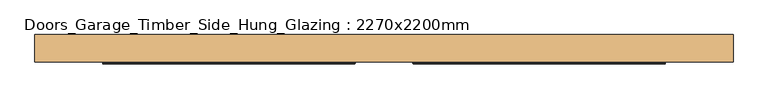
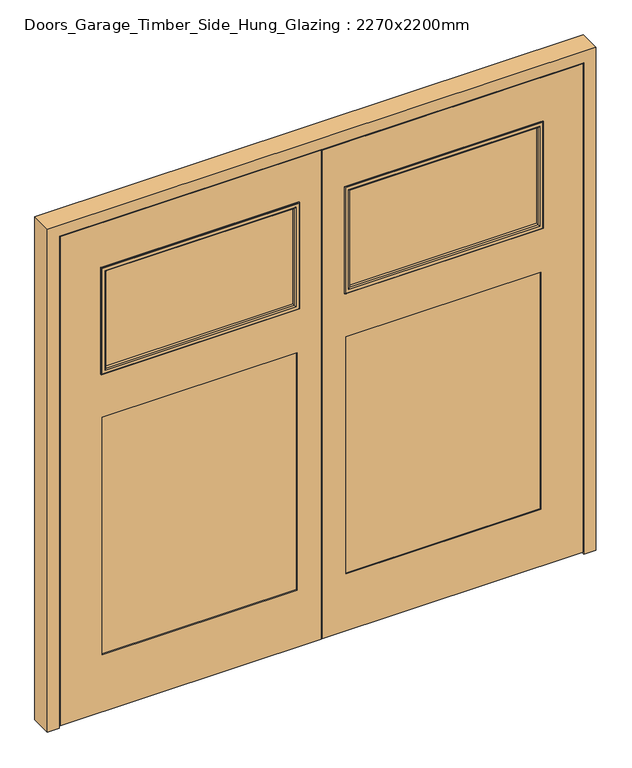
"""IFC4 building model written with IfcOpenShell, lengths in millimetres: door geometry, Doors_Garage_Timber_Side_Hung_Glazing : 2270x2200mm."""

from ifc_helpers import new_model, si_unit, frame, origin, place, context, project, spatial, polyline, ellipse_curve, outline, extrude, faceted_brep, source, transform, mapped, element, save
from ifc_brep_helpers import plane_surface, cylinder_surface, advanced_brep


def doors_garage_timber_side_hung_glazing_2270x2200mm_badb7014(model_context):
    return source(origin(), model_context, "Body", "SolidModel", [
        faceted_brep([(1085.0, -76.6, 0.0), (1085.0, -41.6, 0.0), (1063.0, -41.6, 0.0), (1063.0, 12.4, 0.0), (1135.0, 12.4, 0.0), (1135.0, -76.6, 0.0), (1135.0, -76.6, 2200.0), (-1135.0, -76.6, 2200.0), (-1135.0, -76.6, 0.0), (-1085.0, -76.6, 0.0), (-1085.0, -76.6, 2150.0), (1085.0, -76.6, 2150.0), (1135.0, 12.4, 2200.0), (1063.0, 12.4, 2128.0), (-1063.0, 12.4, 2128.0), (-1063.0, 12.4, 0.0), (-1135.0, 12.4, 0.0), (-1135.0, 12.4, 2200.0), (1063.0, -41.6, 2128.0), (1085.0, -41.6, 2150.0), (-1085.0, -41.6, 2150.0), (-1085.0, -41.6, 0.0), (-1063.0, -41.6, 0.0), (-1063.0, -41.6, 2128.0)], [[[0, 1, 2, 3, 4, 5]], [[5, 6, 7, 8, 9, 10, 11, 0]], [[4, 12, 6, 5]], [[3, 13, 14, 15, 16, 17, 12, 4]], [[2, 18, 13, 3]], [[1, 19, 20, 21, 22, 23, 18, 2]], [[0, 11, 19, 1]], [[9, 21, 20, 10]], [[8, 16, 15, 22, 21, 9]], [[7, 17, 16, 8]], [[14, 23, 22, 15]], [[6, 12, 17, 7]], [[13, 18, 23, 14]], [[10, 20, 19, 11]]]),
        faceted_brep([(1.5, -44.6, 10.0), (1.5, -44.6, 2147.0), (1082.0, -44.6, 2147.0), (1082.0, -44.6, 10.0), (101.5, -44.6, 1947.0), (101.5, -44.6, 1497.0), (907.0, -44.6, 1497.0), (907.0, -44.6, 1947.0), (1.5, -76.6, 10.0), (1082.0, -76.6, 10.0), (1082.0, -76.6, 2147.0), (1.5, -76.6, 2147.0), (101.5, -76.6, 1947.0), (907.0, -76.6, 1947.0), (907.0, -76.6, 1497.0), (101.5, -76.6, 1497.0), (101.5, -76.6, 1297.0), (907.0, -76.6, 1297.0), (907.0, -76.6, 260.0), (101.5, -76.6, 260.0), (101.5, -71.6, 260.0), (907.0, -71.6, 260.0), (907.0, -71.6, 1297.0), (101.5, -71.6, 1297.0)], [[[0, 1, 2, 3], [4, 5, 6, 7]], [[8, 9, 10, 11], [12, 13, 14, 15], [16, 17, 18, 19]], [[3, 9, 8, 0]], [[2, 10, 9, 3]], [[1, 11, 10, 2]], [[0, 8, 11, 1]], [[7, 13, 12, 4]], [[6, 14, 13, 7]], [[5, 15, 14, 6]], [[4, 12, 15, 5]], [[20, 21, 22, 23]], [[23, 16, 19, 20]], [[22, 17, 16, 23]], [[21, 18, 17, 22]], [[20, 19, 18, 21]]]),
        faceted_brep([(-1082.0, -44.6, 10.0), (-1082.0, -44.6, 2147.0), (-1.5, -44.6, 2147.0), (-1.5, -44.6, 10.0), (-101.5, -44.6, 1497.0), (-101.5, -44.6, 1947.0), (-907.0, -44.6, 1947.0), (-907.0, -44.6, 1497.0), (-1082.0, -76.6, 10.0), (-1.5, -76.6, 10.0), (-1.5, -76.6, 2147.0), (-1082.0, -76.6, 2147.0), (-101.5, -76.6, 1497.0), (-907.0, -76.6, 1497.0), (-907.0, -76.6, 1947.0), (-101.5, -76.6, 1947.0), (-101.5, -76.6, 1297.0), (-101.5, -76.6, 260.0), (-907.0, -76.6, 260.0), (-907.0, -76.6, 1297.0), (-907.0, -71.6, 1297.0), (-907.0, -71.6, 260.0), (-101.5, -71.6, 260.0), (-101.5, -71.6, 1297.0)], [[[0, 1, 2, 3], [4, 5, 6, 7]], [[8, 9, 10, 11], [12, 13, 14, 15], [16, 17, 18, 19]], [[3, 9, 8, 0]], [[2, 10, 9, 3]], [[1, 11, 10, 2]], [[0, 8, 11, 1]], [[7, 13, 12, 4]], [[6, 14, 13, 7]], [[5, 15, 14, 6]], [[4, 12, 15, 5]], [[20, 21, 22, 23]], [[23, 16, 19, 20]], [[22, 17, 16, 23]], [[21, 18, 17, 22]], [[20, 19, 18, 21]]]),
        extrude(outline(polyline([(907.0, -54.6), (907.0, -66.6), (101.5, -66.6), (101.5, -54.6), (907.0, -54.6)])), frame((0.0, 0.0, 1497.0), z_axis=(0.0, 0.0, 1.0), x_axis=(1.0, 0.0, 0.0)), (0.0, 0.0, 1.0), 450.0),
        extrude(outline(polyline([(-101.5, -54.6), (-101.5, -66.6), (-907.0, -66.6), (-907.0, -54.6), (-101.5, -54.6)])), frame((0.0, 0.0, 1497.0), z_axis=(0.0, 0.0, 1.0), x_axis=(1.0, 0.0, 0.0)), (0.0, 0.0, 1.0), 450.0),
        advanced_brep(
        [(-907.0, -66.6, 1947.0), (-907.0, -66.6, 1497.0), (-907.0, -76.6, 1497.0), (-907.0, -76.6, 1947.0), (-895.0, -77.6, 1935.0), (-895.0, -77.6, 1509.0), (-895.0, -66.6, 1509.0), (-895.0, -66.6, 1935.0), (-900.0, -82.6, 1940.0), (-900.0, -82.6, 1504.0), (-915.0, -80.6, 1955.0), (-915.0, -80.6, 1489.0), (-913.0, -82.6, 1491.0), (-913.0, -82.6, 1953.0), (-915.0, -76.6, 1955.0), (-915.0, -76.6, 1489.0), (-101.5, -66.6, 1497.0), (-101.5, -76.6, 1497.0), (-113.5, -77.6, 1509.0), (-113.5, -66.6, 1509.0), (-108.5, -82.6, 1504.0), (-93.5, -80.6, 1489.0), (-95.5, -82.6, 1491.0), (-93.5, -76.6, 1489.0), (-101.5, -66.6, 1947.0), (-101.5, -76.6, 1947.0), (-113.5, -77.6, 1935.0), (-113.5, -66.6, 1935.0), (-108.5, -82.6, 1940.0), (-93.5, -80.6, 1955.0), (-95.5, -82.6, 1953.0), (-93.5, -76.6, 1955.0)],
        [
            (0, 1),
            (1, 2),
            (2, 3),
            (3, 0),
            (4, 5),
            (5, 6),
            (6, 7),
            (7, 4),
            (8, 9),
            (9, 5, ellipse_curve(frame((-900.0, -77.6, 1504.0), z_axis=(-0.7071067811865475, 0.0, 0.7071067811865475), x_axis=(0.7071067811865474, 0.0, 0.7071067811865476)), 7.0710678, 5.0)),
            (4, 8, ellipse_curve(frame((-900.0, -77.6, 1940.0), z_axis=(-0.7071067811865475, 0.0, -0.7071067811865475), x_axis=(-0.7071067811865474, 0.0, 0.7071067811865476)), 7.0710678, 5.0)),
            (10, 11),
            (11, 12, ellipse_curve(frame((-913.0, -80.6, 1491.0), z_axis=(-0.7071067811865475, 0.0, 0.7071067811865475), x_axis=(0.7071067811865474, 0.0, 0.7071067811865476)), 2.8284271, 2.0)),
            (12, 13),
            (13, 10, ellipse_curve(frame((-913.0, -80.6, 1953.0), z_axis=(-0.7071067811865475, 0.0, -0.7071067811865475), x_axis=(-0.7071067811865474, 0.0, 0.7071067811865476)), 2.8284271, 2.0)),
            (14, 15),
            (15, 11),
            (10, 14),
            (1, 16),
            (16, 17),
            (17, 2),
            (5, 18),
            (18, 19),
            (19, 6),
            (9, 20),
            (20, 18, ellipse_curve(frame((-108.5, -77.6, 1504.0), z_axis=(-0.7071067811865475, 0.0, -0.7071067811865475), x_axis=(-0.7071067811865476, 0.0, 0.7071067811865474)), 7.0710678, 5.0)),
            (11, 21),
            (21, 22, ellipse_curve(frame((-95.5, -80.6, 1491.0), z_axis=(-0.7071067811865475, 0.0, -0.7071067811865475), x_axis=(-0.7071067811865476, 0.0, 0.7071067811865474)), 2.8284271, 2.0)),
            (22, 12),
            (15, 23),
            (23, 21),
            (16, 24),
            (24, 25),
            (25, 17),
            (18, 26),
            (26, 27),
            (27, 19),
            (20, 28),
            (28, 26, ellipse_curve(frame((-108.5, -77.6, 1940.0), z_axis=(0.7071067811865475, 0.0, -0.7071067811865475), x_axis=(-0.7071067811865474, 0.0, -0.7071067811865476)), 7.0710678, 5.0)),
            (21, 29),
            (29, 30, ellipse_curve(frame((-95.5, -80.6, 1953.0), z_axis=(0.7071067811865475, 0.0, -0.7071067811865475), x_axis=(-0.7071067811865474, 0.0, -0.7071067811865476)), 2.8284271, 2.0)),
            (30, 22),
            (23, 31),
            (31, 29),
            (14, 31),
            (25, 3),
            (24, 0),
            (27, 7),
            (26, 4),
            (28, 8),
            (30, 13),
            (29, 10),
        ],
        [
            plane_surface(frame((-907.0, -76.6, 1947.0), z_axis=(-1.0, 0.0, 0.0), x_axis=(0.0, 0.0, -1.0))),
            plane_surface(frame((-895.0, -66.6, 1935.0), z_axis=(1.0, 0.0, 0.0), x_axis=(0.0, 0.0, -1.0))),
            cylinder_surface(frame((-900.0, -77.6, 1947.0), z_axis=(0.0, 0.0, 1.0), x_axis=(-1.0, 0.0, 0.0)), 5.0),
            cylinder_surface(frame((-913.0, -80.6, 1947.0), z_axis=(0.0, 0.0, 1.0), x_axis=(-1.0, 0.0, 0.0)), 2.0),
            plane_surface(frame((-915.0, -80.6, 1955.0), z_axis=(-1.0, 0.0, 0.0), x_axis=(0.0, 0.0, -1.0))),
            plane_surface(frame((-907.0, -76.6, 1497.0), z_axis=(0.0, 0.0, -1.0), x_axis=(1.0, 0.0, 0.0))),
            plane_surface(frame((-895.0, -66.6, 1509.0), z_axis=(0.0, 0.0, 1.0), x_axis=(1.0, 0.0, 0.0))),
            cylinder_surface(frame((-907.0, -77.6, 1504.0), z_axis=(-1.0, 0.0, 0.0), x_axis=(0.0, 0.0, -1.0)), 5.0),
            cylinder_surface(frame((-907.0, -80.6, 1491.0), z_axis=(-1.0, 0.0, 0.0), x_axis=(0.0, 0.0, -1.0)), 2.0),
            plane_surface(frame((-915.0, -80.6, 1489.0), z_axis=(0.0, 0.0, -1.0), x_axis=(1.0, 0.0, 0.0))),
            plane_surface(frame((-101.5, -76.6, 1497.0), z_axis=(1.0, 0.0, 0.0), x_axis=(0.0, 0.0, 1.0))),
            plane_surface(frame((-113.5, -66.6, 1509.0), z_axis=(-1.0, 0.0, 0.0), x_axis=(0.0, 0.0, 1.0))),
            cylinder_surface(frame((-108.5, -77.6, 1497.0), z_axis=(0.0, 0.0, -1.0), x_axis=(1.0, 0.0, 0.0)), 5.0),
            cylinder_surface(frame((-95.5, -80.6, 1497.0), z_axis=(0.0, 0.0, -1.0), x_axis=(1.0, 0.0, 0.0)), 2.0),
            plane_surface(frame((-93.5, -80.6, 1489.0), z_axis=(1.0, 0.0, 0.0), x_axis=(0.0, 0.0, 1.0))),
            plane_surface(frame((-93.5, -76.6, 1955.0), z_axis=(0.0, 1.0, 0.0), x_axis=(-1.0, 0.0, 0.0))),
            plane_surface(frame((-101.5, -76.6, 1947.0), z_axis=(0.0, 0.0, 1.0), x_axis=(-1.0, 0.0, 0.0))),
            plane_surface(frame((-101.5, -66.6, 1947.0), z_axis=(0.0, 1.0, 0.0), x_axis=(-1.0, 0.0, 0.0))),
            plane_surface(frame((-113.5, -66.6, 1935.0), z_axis=(0.0, 0.0, -1.0), x_axis=(-1.0, 0.0, 0.0))),
            cylinder_surface(frame((-101.5, -77.6, 1940.0), z_axis=(1.0, 0.0, 0.0), x_axis=(0.0, 0.0, 1.0)), 5.0),
            plane_surface(frame((-108.5, -82.6, 1940.0), z_axis=(0.0, -1.0, 0.0), x_axis=(-1.0, 0.0, 0.0))),
            cylinder_surface(frame((-101.5, -80.6, 1953.0), z_axis=(1.0, 0.0, 0.0), x_axis=(0.0, 0.0, 1.0)), 2.0),
            plane_surface(frame((-93.5, -80.6, 1955.0), z_axis=(0.0, 0.0, 1.0), x_axis=(-1.0, 0.0, 0.0))),
        ],
        [
            (0, [[1, 2, 3, 4]]),
            (1, [[5, 6, 7, 8]]),
            (2, [[9, 10, -5, 11]]),
            (3, [[12, 13, 14, 15]]),
            (4, [[16, 17, -12, 18]]),
            (5, [[19, 20, 21, -2]]),
            (6, [[22, 23, 24, -6]]),
            (7, [[25, 26, -22, -10]]),
            (8, [[27, 28, 29, -13]]),
            (9, [[30, 31, -27, -17]]),
            (10, [[32, 33, 34, -20]]),
            (11, [[35, 36, 37, -23]]),
            (12, [[38, 39, -35, -26]]),
            (13, [[40, 41, 42, -28]]),
            (14, [[43, 44, -40, -31]]),
            (15, [[-16, 45, -43, -30], [-3, -21, -34, 46]]),
            (16, [[47, -4, -46, -33]]),
            (17, [[-1, -47, -32, -19], [-7, -24, -37, 48]]),
            (18, [[49, -8, -48, -36]]),
            (19, [[50, -11, -49, -39]]),
            (20, [[-14, -29, -42, 51], [-9, -50, -38, -25]]),
            (21, [[52, -15, -51, -41]]),
            (22, [[-45, -18, -52, -44]]),
        ],
    ),
        advanced_brep(
        [(101.5, -66.6, 1947.0), (101.5, -66.6, 1497.0), (101.5, -76.6, 1497.0), (101.5, -76.6, 1947.0), (113.5, -77.6, 1935.0), (113.5, -77.6, 1509.0), (113.5, -66.6, 1509.0), (113.5, -66.6, 1935.0), (108.5, -82.6, 1940.0), (108.5, -82.6, 1504.0), (93.5, -80.6, 1955.0), (93.5, -80.6, 1489.0), (95.5, -82.6, 1491.0), (95.5, -82.6, 1953.0), (93.5, -76.6, 1955.0), (93.5, -76.6, 1489.0), (907.0, -66.6, 1497.0), (907.0, -76.6, 1497.0), (895.0, -77.6, 1509.0), (895.0, -66.6, 1509.0), (900.0, -82.6, 1504.0), (915.0, -80.6, 1489.0), (913.0, -82.6, 1491.0), (915.0, -76.6, 1489.0), (907.0, -66.6, 1947.0), (907.0, -76.6, 1947.0), (895.0, -77.6, 1935.0), (895.0, -66.6, 1935.0), (900.0, -82.6, 1940.0), (915.0, -80.6, 1955.0), (913.0, -82.6, 1953.0), (915.0, -76.6, 1955.0)],
        [
            (0, 1),
            (1, 2),
            (2, 3),
            (3, 0),
            (4, 5),
            (5, 6),
            (6, 7),
            (7, 4),
            (8, 9),
            (9, 5, ellipse_curve(frame((108.5, -77.6, 1504.0), z_axis=(-0.7071067811865475, 0.0, 0.7071067811865475), x_axis=(0.7071067811865474, 0.0, 0.7071067811865476)), 7.0710678, 5.0)),
            (4, 8, ellipse_curve(frame((108.5, -77.6, 1940.0), z_axis=(-0.7071067811865475, 0.0, -0.7071067811865475), x_axis=(-0.7071067811865474, 0.0, 0.7071067811865476)), 7.0710678, 5.0)),
            (10, 11),
            (11, 12, ellipse_curve(frame((95.5, -80.6, 1491.0), z_axis=(-0.7071067811865475, 0.0, 0.7071067811865475), x_axis=(0.7071067811865474, 0.0, 0.7071067811865476)), 2.8284271, 2.0)),
            (12, 13),
            (13, 10, ellipse_curve(frame((95.5, -80.6, 1953.0), z_axis=(-0.7071067811865475, 0.0, -0.7071067811865475), x_axis=(-0.7071067811865474, 0.0, 0.7071067811865476)), 2.8284271, 2.0)),
            (14, 15),
            (15, 11),
            (10, 14),
            (1, 16),
            (16, 17),
            (17, 2),
            (5, 18),
            (18, 19),
            (19, 6),
            (9, 20),
            (20, 18, ellipse_curve(frame((900.0, -77.6, 1504.0), z_axis=(-0.7071067811865475, 0.0, -0.7071067811865475), x_axis=(-0.7071067811865476, 0.0, 0.7071067811865474)), 7.0710678, 5.0)),
            (11, 21),
            (21, 22, ellipse_curve(frame((913.0, -80.6, 1491.0), z_axis=(-0.7071067811865475, 0.0, -0.7071067811865475), x_axis=(-0.7071067811865476, 0.0, 0.7071067811865474)), 2.8284271, 2.0)),
            (22, 12),
            (15, 23),
            (23, 21),
            (16, 24),
            (24, 25),
            (25, 17),
            (18, 26),
            (26, 27),
            (27, 19),
            (20, 28),
            (28, 26, ellipse_curve(frame((900.0, -77.6, 1940.0), z_axis=(0.7071067811865475, 0.0, -0.7071067811865475), x_axis=(-0.7071067811865474, 0.0, -0.7071067811865476)), 7.0710678, 5.0)),
            (21, 29),
            (29, 30, ellipse_curve(frame((913.0, -80.6, 1953.0), z_axis=(0.7071067811865475, 0.0, -0.7071067811865475), x_axis=(-0.7071067811865474, 0.0, -0.7071067811865476)), 2.8284271, 2.0)),
            (30, 22),
            (23, 31),
            (31, 29),
            (14, 31),
            (25, 3),
            (24, 0),
            (27, 7),
            (26, 4),
            (28, 8),
            (30, 13),
            (29, 10),
        ],
        [
            plane_surface(frame((101.5, -76.6, 1947.0), z_axis=(-1.0, 0.0, 0.0), x_axis=(0.0, 0.0, -1.0))),
            plane_surface(frame((113.5, -66.6, 1935.0), z_axis=(1.0, 0.0, 0.0), x_axis=(0.0, 0.0, -1.0))),
            cylinder_surface(frame((108.5, -77.6, 1947.0), z_axis=(0.0, 0.0, 1.0), x_axis=(-1.0, 0.0, 0.0)), 5.0),
            cylinder_surface(frame((95.5, -80.6, 1947.0), z_axis=(0.0, 0.0, 1.0), x_axis=(-1.0, 0.0, 0.0)), 2.0),
            plane_surface(frame((93.5, -80.6, 1955.0), z_axis=(-1.0, 0.0, 0.0), x_axis=(0.0, 0.0, -1.0))),
            plane_surface(frame((101.5, -76.6, 1497.0), z_axis=(0.0, 0.0, -1.0), x_axis=(1.0, 0.0, 0.0))),
            plane_surface(frame((113.5, -66.6, 1509.0), z_axis=(0.0, 0.0, 1.0), x_axis=(1.0, 0.0, 0.0))),
            cylinder_surface(frame((101.5, -77.6, 1504.0), z_axis=(-1.0, 0.0, 0.0), x_axis=(0.0, 0.0, -1.0)), 5.0),
            cylinder_surface(frame((101.5, -80.6, 1491.0), z_axis=(-1.0, 0.0, 0.0), x_axis=(0.0, 0.0, -1.0)), 2.0),
            plane_surface(frame((93.5, -80.6, 1489.0), z_axis=(0.0, 0.0, -1.0), x_axis=(1.0, 0.0, 0.0))),
            plane_surface(frame((907.0, -76.6, 1497.0), z_axis=(1.0, 0.0, 0.0), x_axis=(0.0, 0.0, 1.0))),
            plane_surface(frame((895.0, -66.6, 1509.0), z_axis=(-1.0, 0.0, 0.0), x_axis=(0.0, 0.0, 1.0))),
            cylinder_surface(frame((900.0, -77.6, 1497.0), z_axis=(0.0, 0.0, -1.0), x_axis=(1.0, 0.0, 0.0)), 5.0),
            cylinder_surface(frame((913.0, -80.6, 1497.0), z_axis=(0.0, 0.0, -1.0), x_axis=(1.0, 0.0, 0.0)), 2.0),
            plane_surface(frame((915.0, -80.6, 1489.0), z_axis=(1.0, 0.0, 0.0), x_axis=(0.0, 0.0, 1.0))),
            plane_surface(frame((915.0, -76.6, 1955.0), z_axis=(0.0, 1.0, 0.0), x_axis=(-1.0, 0.0, 0.0))),
            plane_surface(frame((907.0, -76.6, 1947.0), z_axis=(0.0, 0.0, 1.0), x_axis=(-1.0, 0.0, 0.0))),
            plane_surface(frame((907.0, -66.6, 1947.0), z_axis=(0.0, 1.0, 0.0), x_axis=(-1.0, 0.0, 0.0))),
            plane_surface(frame((895.0, -66.6, 1935.0), z_axis=(0.0, 0.0, -1.0), x_axis=(-1.0, 0.0, 0.0))),
            cylinder_surface(frame((907.0, -77.6, 1940.0), z_axis=(1.0, 0.0, 0.0), x_axis=(0.0, 0.0, 1.0)), 5.0),
            plane_surface(frame((900.0, -82.6, 1940.0), z_axis=(0.0, -1.0, 0.0), x_axis=(-1.0, 0.0, 0.0))),
            cylinder_surface(frame((907.0, -80.6, 1953.0), z_axis=(1.0, 0.0, 0.0), x_axis=(0.0, 0.0, 1.0)), 2.0),
            plane_surface(frame((915.0, -80.6, 1955.0), z_axis=(0.0, 0.0, 1.0), x_axis=(-1.0, 0.0, 0.0))),
        ],
        [
            (0, [[1, 2, 3, 4]]),
            (1, [[5, 6, 7, 8]]),
            (2, [[9, 10, -5, 11]]),
            (3, [[12, 13, 14, 15]]),
            (4, [[16, 17, -12, 18]]),
            (5, [[19, 20, 21, -2]]),
            (6, [[22, 23, 24, -6]]),
            (7, [[25, 26, -22, -10]]),
            (8, [[27, 28, 29, -13]]),
            (9, [[30, 31, -27, -17]]),
            (10, [[32, 33, 34, -20]]),
            (11, [[35, 36, 37, -23]]),
            (12, [[38, 39, -35, -26]]),
            (13, [[40, 41, 42, -28]]),
            (14, [[43, 44, -40, -31]]),
            (15, [[-16, 45, -43, -30], [-3, -21, -34, 46]]),
            (16, [[47, -4, -46, -33]]),
            (17, [[-1, -47, -32, -19], [-7, -24, -37, 48]]),
            (18, [[49, -8, -48, -36]]),
            (19, [[50, -11, -49, -39]]),
            (20, [[-14, -29, -42, 51], [-9, -50, -38, -25]]),
            (21, [[52, -15, -51, -41]]),
            (22, [[-45, -18, -52, -44]]),
        ],
    ),
        advanced_brep(
        [(-101.5, -54.6, 1947.0), (-101.5, -54.6, 1497.0), (-101.5, -44.6, 1497.0), (-101.5, -44.6, 1947.0), (-113.5, -43.6, 1935.0), (-113.5, -43.6, 1509.0), (-113.5, -54.6, 1509.0), (-113.5, -54.6, 1935.0), (-108.5, -38.6, 1940.0), (-108.5, -38.6, 1504.0), (-93.5, -40.6, 1955.0), (-93.5, -40.6, 1489.0), (-95.5, -38.6, 1491.0), (-95.5, -38.6, 1953.0), (-93.5, -44.6, 1955.0), (-93.5, -44.6, 1489.0), (-907.0, -54.6, 1497.0), (-907.0, -44.6, 1497.0), (-895.0, -43.6, 1509.0), (-895.0, -54.6, 1509.0), (-900.0, -38.6, 1504.0), (-915.0, -40.6, 1489.0), (-913.0, -38.6, 1491.0), (-915.0, -44.6, 1489.0), (-907.0, -54.6, 1947.0), (-907.0, -44.6, 1947.0), (-895.0, -43.6, 1935.0), (-895.0, -54.6, 1935.0), (-900.0, -38.6, 1940.0), (-915.0, -40.6, 1955.0), (-913.0, -38.6, 1953.0), (-915.0, -44.6, 1955.0)],
        [
            (0, 1),
            (1, 2),
            (2, 3),
            (3, 0),
            (4, 5),
            (5, 6),
            (6, 7),
            (7, 4),
            (8, 9),
            (9, 5, ellipse_curve(frame((-108.5, -43.6, 1504.0), z_axis=(0.7071067811865426, 0.0, 0.7071067811865525), x_axis=(-0.7071067811865525, 0.0, 0.7071067811865426)), 7.0710678, 5.0)),
            (4, 8, ellipse_curve(frame((-108.5, -43.6, 1940.0), z_axis=(0.7071067811865525, 0.0, -0.7071067811865426), x_axis=(0.7071067811865425, 0.0, 0.7071067811865525)), 7.0710678, 5.0)),
            (10, 11),
            (11, 12, ellipse_curve(frame((-95.5, -40.6, 1491.0), z_axis=(0.7071067811865426, 0.0, 0.7071067811865525), x_axis=(-0.7071067811865525, 0.0, 0.7071067811865426)), 2.8284271, 2.0)),
            (12, 13),
            (13, 10, ellipse_curve(frame((-95.5, -40.6, 1953.0), z_axis=(0.7071067811865525, 0.0, -0.7071067811865426), x_axis=(0.7071067811865425, 0.0, 0.7071067811865525)), 2.8284271, 2.0)),
            (14, 15),
            (15, 11),
            (10, 14),
            (1, 16),
            (16, 17),
            (17, 2),
            (5, 18),
            (18, 19),
            (19, 6),
            (9, 20),
            (20, 18, ellipse_curve(frame((-900.0, -43.6, 1504.0), z_axis=(0.7071067811865527, 0.0, -0.7071067811865422), x_axis=(0.7071067811865424, 0.0, 0.7071067811865527)), 7.0710678, 5.0)),
            (11, 21),
            (21, 22, ellipse_curve(frame((-913.0, -40.6, 1491.0), z_axis=(0.7071067811865527, 0.0, -0.7071067811865422), x_axis=(0.7071067811865424, 0.0, 0.7071067811865527)), 2.8284271, 2.0)),
            (22, 12),
            (15, 23),
            (23, 21),
            (16, 24),
            (24, 25),
            (25, 17),
            (18, 26),
            (26, 27),
            (27, 19),
            (20, 28),
            (28, 26, ellipse_curve(frame((-900.0, -43.6, 1940.0), z_axis=(-0.7071067811865422, 0.0, -0.7071067811865527), x_axis=(0.7071067811865526, 0.0, -0.7071067811865424)), 7.0710678, 5.0)),
            (21, 29),
            (29, 30, ellipse_curve(frame((-913.0, -40.6, 1953.0), z_axis=(-0.7071067811865422, 0.0, -0.7071067811865527), x_axis=(0.7071067811865526, 0.0, -0.7071067811865424)), 2.8284271, 2.0)),
            (30, 22),
            (23, 31),
            (31, 29),
            (14, 31),
            (25, 3),
            (24, 0),
            (27, 7),
            (26, 4),
            (28, 8),
            (30, 13),
            (29, 10),
        ],
        [
            plane_surface(frame((-101.5, -44.6, 1947.0), z_axis=(1.0, 0.0, 0.0), x_axis=(0.0, 0.0, -1.0))),
            plane_surface(frame((-113.5, -54.6, 1935.0), z_axis=(-1.0, 0.0, 0.0), x_axis=(0.0, 0.0, -1.0))),
            cylinder_surface(frame((-108.5, -43.6, 1947.0), z_axis=(0.0, 0.0, 1.0), x_axis=(1.0, 0.0, 0.0)), 5.0),
            cylinder_surface(frame((-95.5, -40.6, 1947.0), z_axis=(0.0, 0.0, 1.0), x_axis=(1.0, 0.0, 0.0)), 2.0),
            plane_surface(frame((-93.5, -40.6, 1955.0), z_axis=(1.0, 0.0, 0.0), x_axis=(0.0, 0.0, -1.0))),
            plane_surface(frame((-101.5, -44.6, 1497.0), z_axis=(0.0, 0.0, -1.0), x_axis=(-1.0, 0.0, 0.0))),
            plane_surface(frame((-113.5, -54.6, 1509.0), z_axis=(0.0, 0.0, 1.0), x_axis=(-1.0, 0.0, 0.0))),
            cylinder_surface(frame((-101.5, -43.6, 1504.0), z_axis=(1.0, 0.0, 0.0), x_axis=(0.0, 0.0, -1.0)), 5.0),
            cylinder_surface(frame((-101.5, -40.6, 1491.0), z_axis=(1.0, 0.0, 0.0), x_axis=(0.0, 0.0, -1.0)), 2.0),
            plane_surface(frame((-93.5, -40.6, 1489.0), z_axis=(0.0, 0.0, -1.0), x_axis=(-1.0, 0.0, 0.0))),
            plane_surface(frame((-907.0, -44.6, 1497.0), z_axis=(-1.0, 0.0, 0.0), x_axis=(0.0, 0.0, 1.0))),
            plane_surface(frame((-895.0, -54.6, 1509.0), z_axis=(1.0, 0.0, 0.0), x_axis=(0.0, 0.0, 1.0))),
            cylinder_surface(frame((-900.0, -43.6, 1497.0), z_axis=(0.0, 0.0, -1.0), x_axis=(-1.0, 0.0, 0.0)), 5.0),
            cylinder_surface(frame((-913.0, -40.6, 1497.0), z_axis=(0.0, 0.0, -1.0), x_axis=(-1.0, 0.0, 0.0)), 2.0),
            plane_surface(frame((-915.0, -40.6, 1489.0), z_axis=(-1.0, 0.0, 0.0), x_axis=(0.0, 0.0, 1.0))),
            plane_surface(frame((-915.0, -44.6, 1955.0), z_axis=(0.0, -1.0, 0.0), x_axis=(1.0, 0.0, 0.0))),
            plane_surface(frame((-907.0, -44.6, 1947.0), z_axis=(0.0, 0.0, 1.0), x_axis=(1.0, 0.0, 0.0))),
            plane_surface(frame((-907.0, -54.6, 1947.0), z_axis=(0.0, -1.0, 0.0), x_axis=(1.0, 0.0, 0.0))),
            plane_surface(frame((-895.0, -54.6, 1935.0), z_axis=(0.0, 0.0, -1.0), x_axis=(1.0, 0.0, 0.0))),
            cylinder_surface(frame((-907.0, -43.6, 1940.0), z_axis=(-1.0, 0.0, 0.0), x_axis=(0.0, 0.0, 1.0)), 5.0),
            plane_surface(frame((-900.0, -38.6, 1940.0), z_axis=(0.0, 1.0, 0.0), x_axis=(1.0, 0.0, 0.0))),
            cylinder_surface(frame((-907.0, -40.6, 1953.0), z_axis=(-1.0, 0.0, 0.0), x_axis=(0.0, 0.0, 1.0)), 2.0),
            plane_surface(frame((-915.0, -40.6, 1955.0), z_axis=(0.0, 0.0, 1.0), x_axis=(1.0, 0.0, 0.0))),
        ],
        [
            (0, [[1, 2, 3, 4]]),
            (1, [[5, 6, 7, 8]]),
            (2, [[9, 10, -5, 11]]),
            (3, [[12, 13, 14, 15]]),
            (4, [[16, 17, -12, 18]]),
            (5, [[19, 20, 21, -2]]),
            (6, [[22, 23, 24, -6]]),
            (7, [[25, 26, -22, -10]]),
            (8, [[27, 28, 29, -13]]),
            (9, [[30, 31, -27, -17]]),
            (10, [[32, 33, 34, -20]]),
            (11, [[35, 36, 37, -23]]),
            (12, [[38, 39, -35, -26]]),
            (13, [[40, 41, 42, -28]]),
            (14, [[43, 44, -40, -31]]),
            (15, [[-16, 45, -43, -30], [-3, -21, -34, 46]]),
            (16, [[47, -4, -46, -33]]),
            (17, [[-1, -47, -32, -19], [-7, -24, -37, 48]]),
            (18, [[49, -8, -48, -36]]),
            (19, [[50, -11, -49, -39]]),
            (20, [[-14, -29, -42, 51], [-9, -50, -38, -25]]),
            (21, [[52, -15, -51, -41]]),
            (22, [[-45, -18, -52, -44]]),
        ],
    ),
        advanced_brep(
        [(907.0, -54.6, 1947.0), (907.0, -54.6, 1497.0), (907.0, -44.6, 1497.0), (907.0, -44.6, 1947.0), (895.0, -43.6, 1935.0), (895.0, -43.6, 1509.0), (895.0, -54.6, 1509.0), (895.0, -54.6, 1935.0), (900.0, -38.6, 1940.0), (900.0, -38.6, 1504.0), (915.0, -40.6, 1955.0), (915.0, -40.6, 1489.0), (913.0, -38.6, 1491.0), (913.0, -38.6, 1953.0), (915.0, -44.6, 1955.0), (915.0, -44.6, 1489.0), (101.5, -54.6, 1497.0), (101.5, -44.6, 1497.0), (113.5, -43.6, 1509.0), (113.5, -54.6, 1509.0), (108.5, -38.6, 1504.0), (93.5, -40.6, 1489.0), (95.5, -38.6, 1491.0), (93.5, -44.6, 1489.0), (101.5, -54.6, 1947.0), (101.5, -44.6, 1947.0), (113.5, -43.6, 1935.0), (113.5, -54.6, 1935.0), (108.5, -38.6, 1940.0), (93.5, -40.6, 1955.0), (95.5, -38.6, 1953.0), (93.5, -44.6, 1955.0)],
        [
            (0, 1),
            (1, 2),
            (2, 3),
            (3, 0),
            (4, 5),
            (5, 6),
            (6, 7),
            (7, 4),
            (8, 9),
            (9, 5, ellipse_curve(frame((900.0, -43.6, 1504.0), z_axis=(0.7071067811865424, 0.0, 0.7071067811865527), x_axis=(-0.7071067811865527, 0.0, 0.7071067811865422)), 7.0710678, 5.0)),
            (4, 8, ellipse_curve(frame((900.0, -43.6, 1940.0), z_axis=(0.7071067811865528, 0.0, -0.7071067811865422), x_axis=(0.7071067811865422, 0.0, 0.7071067811865528)), 7.0710678, 5.0)),
            (10, 11),
            (11, 12, ellipse_curve(frame((913.0, -40.6, 1491.0), z_axis=(0.7071067811865424, 0.0, 0.7071067811865527), x_axis=(-0.7071067811865527, 0.0, 0.7071067811865422)), 2.8284271, 2.0)),
            (12, 13),
            (13, 10, ellipse_curve(frame((913.0, -40.6, 1953.0), z_axis=(0.7071067811865528, 0.0, -0.7071067811865422), x_axis=(0.7071067811865422, 0.0, 0.7071067811865528)), 2.8284271, 2.0)),
            (14, 15),
            (15, 11),
            (10, 14),
            (1, 16),
            (16, 17),
            (17, 2),
            (5, 18),
            (18, 19),
            (19, 6),
            (9, 20),
            (20, 18, ellipse_curve(frame((108.5, -43.6, 1504.0), z_axis=(0.7071067811865528, 0.0, -0.7071067811865424), x_axis=(0.7071067811865421, 0.0, 0.7071067811865528)), 7.0710678, 5.0)),
            (11, 21),
            (21, 22, ellipse_curve(frame((95.5, -40.6, 1491.0), z_axis=(0.7071067811865528, 0.0, -0.7071067811865424), x_axis=(0.7071067811865421, 0.0, 0.7071067811865528)), 2.8284271, 2.0)),
            (22, 12),
            (15, 23),
            (23, 21),
            (16, 24),
            (24, 25),
            (25, 17),
            (18, 26),
            (26, 27),
            (27, 19),
            (20, 28),
            (28, 26, ellipse_curve(frame((108.5, -43.6, 1940.0), z_axis=(-0.7071067811865422, 0.0, -0.7071067811865528), x_axis=(0.7071067811865527, 0.0, -0.7071067811865424)), 7.0710678, 5.0)),
            (21, 29),
            (29, 30, ellipse_curve(frame((95.5, -40.6, 1953.0), z_axis=(-0.7071067811865422, 0.0, -0.7071067811865528), x_axis=(0.7071067811865527, 0.0, -0.7071067811865424)), 2.8284271, 2.0)),
            (30, 22),
            (23, 31),
            (31, 29),
            (14, 31),
            (25, 3),
            (24, 0),
            (27, 7),
            (26, 4),
            (28, 8),
            (30, 13),
            (29, 10),
        ],
        [
            plane_surface(frame((907.0, -44.6, 1947.0), z_axis=(1.0, 0.0, 0.0), x_axis=(0.0, 0.0, -1.0))),
            plane_surface(frame((895.0, -54.6, 1935.0), z_axis=(-1.0, 0.0, 0.0), x_axis=(0.0, 0.0, -1.0))),
            cylinder_surface(frame((900.0, -43.6, 1947.0), z_axis=(0.0, 0.0, 1.0), x_axis=(1.0, 0.0, 0.0)), 5.0),
            cylinder_surface(frame((913.0, -40.6, 1947.0), z_axis=(0.0, 0.0, 1.0), x_axis=(1.0, 0.0, 0.0)), 2.0),
            plane_surface(frame((915.0, -40.6, 1955.0), z_axis=(1.0, 0.0, 0.0), x_axis=(0.0, 0.0, -1.0))),
            plane_surface(frame((907.0, -44.6, 1497.0), z_axis=(0.0, 0.0, -1.0), x_axis=(-1.0, 0.0, 0.0))),
            plane_surface(frame((895.0, -54.6, 1509.0), z_axis=(0.0, 0.0, 1.0), x_axis=(-1.0, 0.0, 0.0))),
            cylinder_surface(frame((907.0, -43.6, 1504.0), z_axis=(1.0, 0.0, 0.0), x_axis=(0.0, 0.0, -1.0)), 5.0),
            cylinder_surface(frame((907.0, -40.6, 1491.0), z_axis=(1.0, 0.0, 0.0), x_axis=(0.0, 0.0, -1.0)), 2.0),
            plane_surface(frame((915.0, -40.6, 1489.0), z_axis=(0.0, 0.0, -1.0), x_axis=(-1.0, 0.0, 0.0))),
            plane_surface(frame((101.5, -44.6, 1497.0), z_axis=(-1.0, 0.0, 0.0), x_axis=(0.0, 0.0, 1.0))),
            plane_surface(frame((113.5, -54.6, 1509.0), z_axis=(1.0, 0.0, 0.0), x_axis=(0.0, 0.0, 1.0))),
            cylinder_surface(frame((108.5, -43.6, 1497.0), z_axis=(0.0, 0.0, -1.0), x_axis=(-1.0, 0.0, 0.0)), 5.0),
            cylinder_surface(frame((95.5, -40.6, 1497.0), z_axis=(0.0, 0.0, -1.0), x_axis=(-1.0, 0.0, 0.0)), 2.0),
            plane_surface(frame((93.5, -40.6, 1489.0), z_axis=(-1.0, 0.0, 0.0), x_axis=(0.0, 0.0, 1.0))),
            plane_surface(frame((93.5, -44.6, 1955.0), z_axis=(0.0, -1.0, 0.0), x_axis=(1.0, 0.0, 0.0))),
            plane_surface(frame((101.5, -44.6, 1947.0), z_axis=(0.0, 0.0, 1.0), x_axis=(1.0, 0.0, 0.0))),
            plane_surface(frame((101.5, -54.6, 1947.0), z_axis=(0.0, -1.0, 0.0), x_axis=(1.0, 0.0, 0.0))),
            plane_surface(frame((113.5, -54.6, 1935.0), z_axis=(0.0, 0.0, -1.0), x_axis=(1.0, 0.0, 0.0))),
            cylinder_surface(frame((101.5, -43.6, 1940.0), z_axis=(-1.0, 0.0, 0.0), x_axis=(0.0, 0.0, 1.0)), 5.0),
            plane_surface(frame((108.5, -38.6, 1940.0), z_axis=(0.0, 1.0, 0.0), x_axis=(1.0, 0.0, 0.0))),
            cylinder_surface(frame((101.5, -40.6, 1953.0), z_axis=(-1.0, 0.0, 0.0), x_axis=(0.0, 0.0, 1.0)), 2.0),
            plane_surface(frame((93.5, -40.6, 1955.0), z_axis=(0.0, 0.0, 1.0), x_axis=(1.0, 0.0, 0.0))),
        ],
        [
            (0, [[1, 2, 3, 4]]),
            (1, [[5, 6, 7, 8]]),
            (2, [[9, 10, -5, 11]]),
            (3, [[12, 13, 14, 15]]),
            (4, [[16, 17, -12, 18]]),
            (5, [[19, 20, 21, -2]]),
            (6, [[22, 23, 24, -6]]),
            (7, [[25, 26, -22, -10]]),
            (8, [[27, 28, 29, -13]]),
            (9, [[30, 31, -27, -17]]),
            (10, [[32, 33, 34, -20]]),
            (11, [[35, 36, 37, -23]]),
            (12, [[38, 39, -35, -26]]),
            (13, [[40, 41, 42, -28]]),
            (14, [[43, 44, -40, -31]]),
            (15, [[-16, 45, -43, -30], [-3, -21, -34, 46]]),
            (16, [[47, -4, -46, -33]]),
            (17, [[-1, -47, -32, -19], [-7, -24, -37, 48]]),
            (18, [[49, -8, -48, -36]]),
            (19, [[50, -11, -49, -39]]),
            (20, [[-14, -29, -42, 51], [-9, -50, -38, -25]]),
            (21, [[52, -15, -51, -41]]),
            (22, [[-45, -18, -52, -44]]),
        ],
    ),
    ])


if __name__ == "__main__":
    model = new_model("IFC4")
    model_context = context("Model", 3, world=origin())
    ifc_project = project(units=[si_unit("LENGTHUNIT", "METRE", prefix="MILLI")], contexts=[model_context])
    site = spatial("IfcSite", under=ifc_project)
    building = spatial("IfcBuilding", under=site)
    placement = place(None, origin())
    doors_garage_timber_side_hung_glazing_2270x2200mm_shape = doors_garage_timber_side_hung_glazing_2270x2200mm_badb7014(model_context)
    element("IfcDoor", 1, ObjectType="Doors_Garage_Timber_Side_Hung_Glazing : 2270x2200mm", at=placement, inside=building, context=model_context, shape_type="MappedRepresentation", body=[
        mapped(doors_garage_timber_side_hung_glazing_2270x2200mm_shape, transform((0.0, 0.0, 0.0), x_axis=(1.0, 0.0, 0.0), y_axis=(0.0, 1.0, 0.0), z_axis=(0.0, 0.0, 1.0))),
    ])
    save(model, "model.ifc")

# Revit data of these elements
# Type "Doors_Garage_Timber_Side_Hung_Glazing : 2270x2200mm"
#   Type Mark = "9"
#   Type Comments = "External Garage"
#   Operation = "DoubleDoorSingleSwing"
#   Construction Type Id = "GSP4R"
#   Manufacturer = "Revit"
#   Keynote = "L20"
#   Analytic Construction = "1/8 in Pilkington single glazing"
#   Wrap Layers (Ext) from Ext = 0' - 4.03543"
#   Wrap Layers (Int) from Ext = 0' - 6.98819"
#   Visual Light Transmittance = 0.9
#   Thickness = 0' - 1.25984"
#   Stile Top Rail = 0' - 7.87402"
#   Stile Shutting = 0' - 3.93701"
#   Stile Lock Rail = 0' - 7.87402"
#   Stile Hanging = 0' - 6.88976"
#   Stile Bottom Rail = 0' - 9.84252"
#   Solar Heat Gain Coefficient = 0.78
#   Rough Width = 7' - 5.37008"
#   Rough Height = 7' - 2.61417"
#   O/A Frame Width = 0' - 2.51969"
#   Heat Transfer Coefficient (U) = 0.6496 BTU/(h·ft²·°F)
#   Handle Z Distance = 3' - 5.33858"
#   Glazing Panel Height = 1' - 5.71654"
#   FrameWidth = 0' - 1.65354"
#   FrameOffset - External = 0' - 0.98425"
#   FrameDepth = 0' - 3.50394"
#   Door Panel Thickness = 0' - 1.25984"
#   Height = 7' - 2.61417"
#   Structural Tolerance = 0' - 0.31496"
#   Tolerance = 0' - 0.11811"
#   Undercut = 0' - 0.3937"
#   Width = 7' - 5.37008"
#   Cavity Closer Width = 0' - 1.9685"
#   Cavity Closer Offset from Ext = 0' - 4.03543"
#   Cavity Closer Depth = 0' - 3.34646"
#   Vis - Cavity Closers = yes
#   Define Thermal Properties by = 1
#   Function = 1
#   Material Door = Door - Panel
#   Material Frame = Door - Frame/Mullion
#   Material Ironmongery = Door - Handle
#   Wall Closure = (empty or 0)
# Element 1 (IfcDoor, "Doors_Garage_Timber_Side_Hung_Glazing : 2270x2200mm")
#   Materials on its faces: "Door - Panel", "Door - Frame/Mullion", "Door - Glazing"
# Materials
#   "Door - Panel": class "Wood", colour RGB 210 159 95, transparency 0, Cost = 0
#   "Door - Frame/Mullion": class "Wood", colour RGB 212 179 113, transparency 0
#   "Door - Handle": colour RGB 0 0 0, transparency 0
#   "Door - Glazing": colour RGB 0 0 255, transparency 0.75
